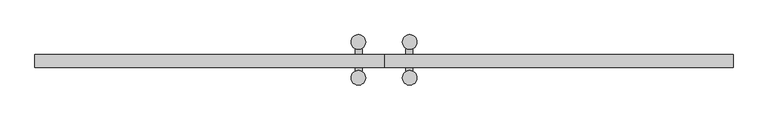
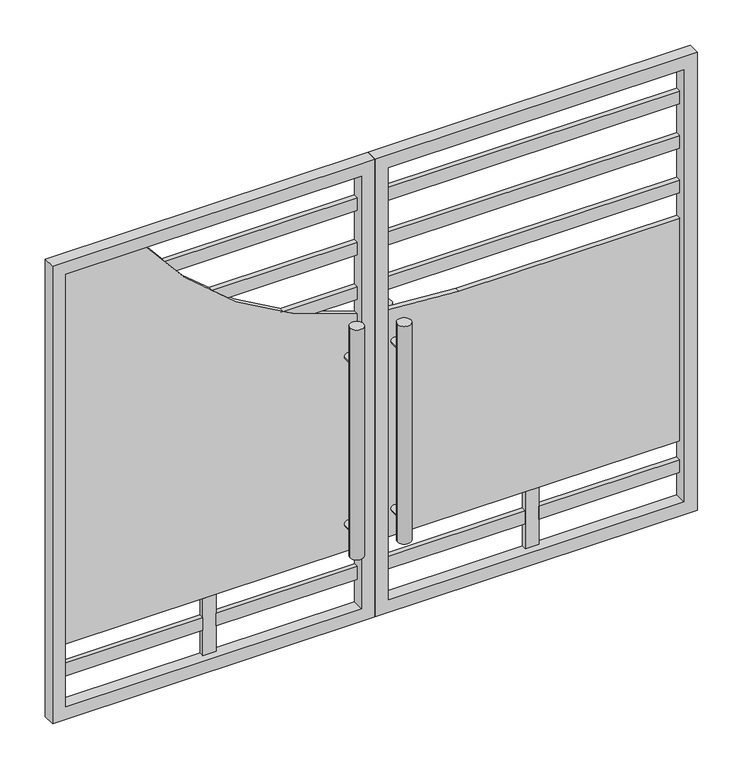
"""IFC4 building model written with IfcOpenShell, lengths in millimetres: proxy geometry."""

from ifc_helpers import new_model, si_unit, point, frame, frame_2d, origin, place, context, project, spatial, polyline, circle_curve, trimmed, segment, composite_curve, outline, extrude, source, transform, mapped, element, save


def generic_models_113f6068(model_context):
    return source(origin(), model_context, "Body", "SweptSolid", [
        extrude(outline(polyline([(0.0, -1219.2), (0.0, 0.0), (1828.8, 0.0), (1828.8, -1219.2), (0.0, -1219.2)]), holes=[polyline([(50.8, -1168.4), (1778.0, -1168.4), (1778.0, -50.8), (50.8, -50.8), (50.8, -1168.4)])]), frame((0.0, -46.0617726, 0.0), z_axis=(0.0, 1.0, 0.0), x_axis=(0.0, 0.0, 1.0)), (0.0, 0.0, 1.0), 46.0617726),
        extrude(outline(polyline([(0.0, 1219.2), (1828.8, 1219.2), (1828.8, 0.0), (0.0, 0.0), (0.0, 1219.2)]), holes=[polyline([(50.8, 1168.4), (50.8, 50.8), (1778.0, 50.8), (1778.0, 1168.4), (50.8, 1168.4)])]), frame((0.0, -46.0617726, 0.0), z_axis=(0.0, 1.0, 0.0), x_axis=(0.0, 0.0, 1.0)), (0.0, 0.0, 1.0), 46.0617726),
        extrude(outline(composite_curve([segment(polyline([(1778.0, -1168.4), (279.4, -1168.4), (279.4, -50.8), (1212.1744192, -50.8)]), True, "CONTINUOUS"), segment(trimmed(circle_curve(frame_2d((2582.6324877, 299.8877691)), 1414.6155764), [point((1212.1744192, -50.8))], [point((1778.0, -863.6))], True, "CARTESIAN"), True, "CONTINUOUS"), segment(polyline([(1778.0, -863.6), (1778.0, -1168.4)]), True, "CONTINUOUS")], self_intersect=False)), frame((0.0, -19.05, 0.0), z_axis=(0.0, 1.0, 0.0), x_axis=(0.0, 0.0, 1.0)), (0.0, 0.0, 1.0), 19.05),
        extrude(outline(composite_curve([segment(polyline([(279.4, 1168.4), (1168.4, 1168.4), (1168.4, 332.8073642)]), True, "CONTINUOUS"), segment(trimmed(circle_curve(frame_2d((2582.6324877, 299.8877691)), 1414.6155764), [point((1168.4, 332.8073642))], [point((1190.1194672, 50.8))], True, "CARTESIAN"), True, "CONTINUOUS"), segment(polyline([(1190.1194672, 50.8), (279.4, 50.8), (279.4, 1168.4)]), True, "CONTINUOUS")], self_intersect=False)), frame((0.0, -19.05, 0.0), z_axis=(0.0, 1.0, 0.0), x_axis=(0.0, 0.0, 1.0)), (0.0, 0.0, 1.0), 19.05),
        extrude(outline(composite_curve([segment(polyline([(1676.4, -50.8), (1676.4, -786.3350015)]), True, "CONTINUOUS"), segment(trimmed(circle_curve(frame_2d((2582.6324877, 299.8877691)), 1414.6155764), [point((1676.4, -786.3350015))], [point((1625.6, -741.8540639))], False, "CARTESIAN"), True, "CONTINUOUS"), segment(polyline([(1625.6, -741.8540639), (1625.6, -50.8), (1676.4, -50.8)]), True, "CONTINUOUS")], self_intersect=False)), frame((0.0, -19.05, 0.0), z_axis=(0.0, 1.0, 0.0), x_axis=(0.0, 0.0, 1.0)), (0.0, 0.0, 1.0), 19.05),
        extrude(outline(polyline([(1171.575, -19.05), (50.8, -19.05), (50.8, 0.0), (1171.575, 0.0), (1171.575, -19.05)])), frame((0.0, 0.0, 1625.6), z_axis=(0.0, 0.0, 1.0), x_axis=(1.0, 0.0, 0.0)), (0.0, 0.0, 1.0), 50.8),
        extrude(outline(composite_curve([segment(polyline([(1498.6, -50.8), (1498.6, -608.963591)]), True, "CONTINUOUS"), segment(trimmed(circle_curve(frame_2d((2582.6324877, 299.8877691)), 1414.6155764), [point((1498.6, -608.963591))], [point((1447.8, -544.6786605))], False, "CARTESIAN"), True, "CONTINUOUS"), segment(polyline([(1447.8, -544.6786605), (1447.8, -50.8), (1498.6, -50.8)]), True, "CONTINUOUS")], self_intersect=False)), frame((0.0, -19.05, 0.0), z_axis=(0.0, 1.0, 0.0), x_axis=(0.0, 0.0, 1.0)), (0.0, 0.0, 1.0), 19.05),
        extrude(outline(polyline([(1171.575, -19.05), (50.8, -19.05), (50.8, 0.0), (1171.575, 0.0), (1171.575, -19.05)])), frame((0.0, 0.0, 1447.8), z_axis=(0.0, 0.0, 1.0), x_axis=(1.0, 0.0, 0.0)), (0.0, 0.0, 1.0), 50.8),
        extrude(outline(composite_curve([segment(polyline([(1320.8, -50.8), (1320.8, -339.5776342)]), True, "CONTINUOUS"), segment(trimmed(circle_curve(frame_2d((2582.6324877, 299.8877691)), 1414.6155764), [point((1320.8, -339.5776342))], [point((1270.0, -227.4955652))], False, "CARTESIAN"), True, "CONTINUOUS"), segment(polyline([(1270.0, -227.4955652), (1270.0, -50.8), (1320.8, -50.8)]), True, "CONTINUOUS")], self_intersect=False)), frame((0.0, -19.05, 0.0), z_axis=(0.0, 1.0, 0.0), x_axis=(0.0, 0.0, 1.0)), (0.0, 0.0, 1.0), 19.05),
        extrude(outline(polyline([(1171.575, -19.05), (50.8, -19.05), (50.8, 0.0), (1171.575, 0.0), (1171.575, -19.05)])), frame((0.0, 0.0, 1270.0), z_axis=(0.0, 0.0, 1.0), x_axis=(1.0, 0.0, 0.0)), (0.0, 0.0, 1.0), 50.8),
        extrude(outline(polyline([(-635.0, -19.05), (-1168.4, -19.05), (-1168.4, 0.0), (-635.0, 0.0), (-635.0, -19.05)])), frame((0.0, 0.0, 152.4), z_axis=(0.0, 0.0, 1.0), x_axis=(1.0, 0.0, 0.0)), (0.0, 0.0, 1.0), 50.8),
        extrude(outline(polyline([(-50.8, -19.05), (-584.2, -19.05), (-584.2, 0.0), (-50.8, 0.0), (-50.8, -19.05)])), frame((0.0, 0.0, 152.4), z_axis=(0.0, 0.0, 1.0), x_axis=(1.0, 0.0, 0.0)), (0.0, 0.0, 1.0), 50.8),
        extrude(outline(polyline([(1168.4, -19.05), (635.0, -19.05), (635.0, 0.0), (1168.4, 0.0), (1168.4, -19.05)])), frame((0.0, 0.0, 152.4), z_axis=(0.0, 0.0, 1.0), x_axis=(1.0, 0.0, 0.0)), (0.0, 0.0, 1.0), 50.8),
        extrude(outline(polyline([(584.2, -19.05), (50.8, -19.05), (50.8, 0.0), (584.2, 0.0), (584.2, -19.05)])), frame((0.0, 0.0, 152.4), z_axis=(0.0, 0.0, 1.0), x_axis=(1.0, 0.0, 0.0)), (0.0, 0.0, 1.0), 50.8),
        extrude(outline(polyline([(-584.2, -19.05), (-635.0, -19.05), (-635.0, 0.0), (-584.2, 0.0), (-584.2, -19.05)])), frame((0.0, 0.0, 50.8), z_axis=(0.0, 0.0, 1.0), x_axis=(1.0, 0.0, 0.0)), (0.0, 0.0, 1.0), 228.6),
        extrude(outline(polyline([(635.0, -19.05), (584.2, -19.05), (584.2, 0.0), (635.0, 0.0), (635.0, -19.05)])), frame((0.0, 0.0, 50.8), z_axis=(0.0, 0.0, 1.0), x_axis=(1.0, 0.0, 0.0)), (0.0, 0.0, 1.0), 228.6),
        extrude(outline(composite_curve([segment(trimmed(circle_curve(frame_2d((-89.7949058, 43.7785099)), 25.4), [point((-64.3949058, 43.7785099))], [point((-115.1949058, 43.7785099))], False, "CARTESIAN"), True, "CONTINUOUS"), segment(trimmed(circle_curve(frame_2d((-89.7949058, 43.7785099)), 25.4), [point((-115.1949058, 43.7785099))], [point((-64.3949058, 43.7785099))], False, "CARTESIAN"), True, "CONTINUOUS")], self_intersect=False)), frame((0.0, 0.0, 279.4), z_axis=(0.0, 0.0, 1.0), x_axis=(1.0, 0.0, 0.0)), (0.0, 0.0, 1.0), 889.0),
        extrude(outline(composite_curve([segment(trimmed(circle_curve(frame_2d((89.7949058, 43.7785099)), 25.4), [point((64.3949058, 43.7785099))], [point((115.1949058, 43.7785099))], False, "CARTESIAN"), True, "CONTINUOUS"), segment(trimmed(circle_curve(frame_2d((89.7949058, 43.7785099)), 25.4), [point((115.1949058, 43.7785099))], [point((64.3949058, 43.7785099))], False, "CARTESIAN"), True, "CONTINUOUS")], self_intersect=False)), frame((0.0, 0.0, 279.4), z_axis=(0.0, 0.0, 1.0), x_axis=(1.0, 0.0, 0.0)), (0.0, 0.0, 1.0), 889.0),
        extrude(outline(composite_curve([segment(trimmed(circle_curve(frame_2d((-89.7949058, -81.8785099)), 25.4), [point((-64.3949058, -81.8785099))], [point((-115.1949058, -81.8785099))], False, "CARTESIAN"), True, "CONTINUOUS"), segment(trimmed(circle_curve(frame_2d((-89.7949058, -81.8785099)), 25.4), [point((-115.1949058, -81.8785099))], [point((-64.3949058, -81.8785099))], False, "CARTESIAN"), True, "CONTINUOUS")], self_intersect=False)), frame((0.0, 0.0, 298.8472671), z_axis=(0.0, 0.0, 1.0), x_axis=(1.0, 0.0, 0.0)), (0.0, 0.0, 1.0), 917.3073645),
        extrude(outline(composite_curve([segment(trimmed(circle_curve(frame_2d((89.7949058, -81.8785099)), 25.4), [point((64.3949058, -81.8785099))], [point((115.1949058, -81.8785099))], False, "CARTESIAN"), True, "CONTINUOUS"), segment(trimmed(circle_curve(frame_2d((89.7949058, -81.8785099)), 25.4), [point((115.1949058, -81.8785099))], [point((64.3949058, -81.8785099))], False, "CARTESIAN"), True, "CONTINUOUS")], self_intersect=False)), frame((0.0, 0.0, 298.8472671), z_axis=(0.0, 0.0, 1.0), x_axis=(1.0, 0.0, 0.0)), (0.0, 0.0, 1.0), 869.5527329),
        extrude(outline(composite_curve([segment(trimmed(circle_curve(frame_2d((1058.3458504, 88.119132)), 12.7), [point((1058.3458504, 75.419132))], [point((1058.3458504, 100.819132))], False, "CARTESIAN"), True, "CONTINUOUS"), segment(trimmed(circle_curve(frame_2d((1058.3458504, 88.119132)), 12.7), [point((1058.3458504, 100.819132))], [point((1058.3458504, 75.419132))], False, "CARTESIAN"), True, "CONTINUOUS")], self_intersect=False)), frame((0.0, -57.15, 0.0), z_axis=(0.0, 1.0, 0.0), x_axis=(0.0, 0.0, 1.0)), (0.0, 0.0, 1.0), 76.6172039),
        extrude(outline(composite_curve([segment(trimmed(circle_curve(frame_2d((389.4541496, 88.119132)), 12.7), [point((389.4541496, 75.419132))], [point((389.4541496, 100.819132))], False, "CARTESIAN"), True, "CONTINUOUS"), segment(trimmed(circle_curve(frame_2d((389.4541496, 88.119132)), 12.7), [point((389.4541496, 100.819132))], [point((389.4541496, 75.419132))], False, "CARTESIAN"), True, "CONTINUOUS")], self_intersect=False)), frame((0.0, -57.15, 0.0), z_axis=(0.0, 1.0, 0.0), x_axis=(0.0, 0.0, 1.0)), (0.0, 0.0, 1.0), 76.7981605),
        extrude(outline(composite_curve([segment(trimmed(circle_curve(frame_2d((1058.3458504, -88.119132)), 12.7), [point((1058.3458504, -75.419132))], [point((1058.3458504, -100.819132))], False, "CARTESIAN"), True, "CONTINUOUS"), segment(trimmed(circle_curve(frame_2d((1058.3458504, -88.119132)), 12.7), [point((1058.3458504, -100.819132))], [point((1058.3458504, -75.419132))], False, "CARTESIAN"), True, "CONTINUOUS")], self_intersect=False)), frame((0.0, -57.15, 0.0), z_axis=(0.0, 1.0, 0.0), x_axis=(0.0, 0.0, 1.0)), (0.0, 0.0, 1.0), 76.6172039),
        extrude(outline(composite_curve([segment(trimmed(circle_curve(frame_2d((389.4541496, -88.119132)), 12.7), [point((389.4541496, -75.419132))], [point((389.4541496, -100.819132))], False, "CARTESIAN"), True, "CONTINUOUS"), segment(trimmed(circle_curve(frame_2d((389.4541496, -88.119132)), 12.7), [point((389.4541496, -100.819132))], [point((389.4541496, -75.419132))], False, "CARTESIAN"), True, "CONTINUOUS")], self_intersect=False)), frame((0.0, -57.15, 0.0), z_axis=(0.0, 1.0, 0.0), x_axis=(0.0, 0.0, 1.0)), (0.0, 0.0, 1.0), 76.7981605),
    ])


if __name__ == "__main__":
    model = new_model("IFC4")
    model_context = context("Model", 3, world=origin())
    ifc_project = project(units=[si_unit("LENGTHUNIT", "METRE", prefix="MILLI")], contexts=[model_context])
    site = spatial("IfcSite", under=ifc_project)
    building = spatial("IfcBuilding", under=site)
    placement = place(None, origin())
    generic_models_shape = generic_models_113f6068(model_context)
    element("IfcBuildingElementProxy", 1, Name="Generic Models", at=placement, inside=building, context=model_context, shape_type="MappedRepresentation", body=[
        mapped(generic_models_shape, transform((0.0, 0.0, 0.0), x_axis=(1.0, 0.0, 0.0), y_axis=(0.0, 1.0, 0.0), z_axis=(0.0, 0.0, 1.0))),
    ])
    save(model, "model.ifc")

# Revit data of these elements
# Type
#   sheet = none
#   pipe = none
#   handal = none
#   faram = none
#   Default Elevation = 0
